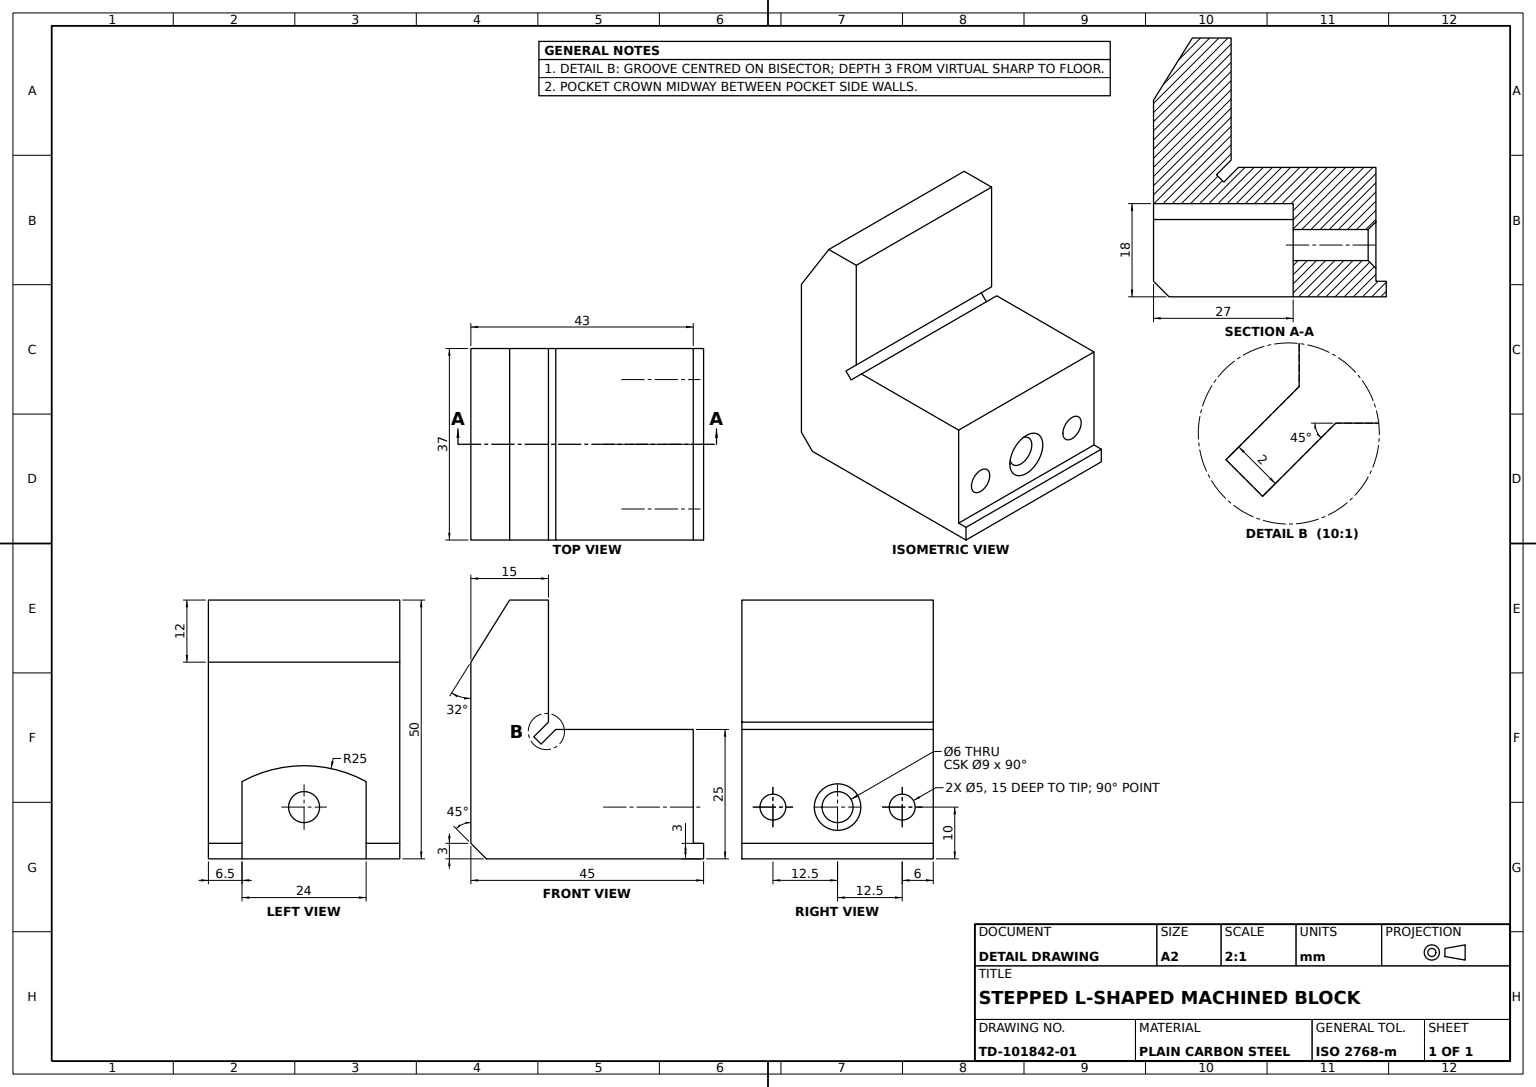
SolidWorks part; units mm, degrees
material "Plain Carbon Steel"
ref_plane "Front Plane" through (0, 0, 0) normal (0, 0, 1) x (1, 0, 0)
ref_plane "Top Plane" through (0, 0, 0) normal (0, 1, 0) x (1, 0, 0)
ref_plane "Right Plane" through (0, 0, 0) normal (1, 0, 0) x (0, 0, -1)
sketch "Block Profile Sketch" plane through (0, 0, 0) normal (0, 0, 1) x (1, 0, 0)
  line L0 (0, 0) -> (0, 13)
  line L1 (0, 13) -> (7.4984, 25)
  line L2 (7.4984, 25) -> (15, 25)
  line L3 (15, 25) -> (15, 0)
  line L4 (15, 0) -> (43, 0)
  line L5 (43, 0) -> (43, -22)
  line L6 (43, -22) -> (45, -22)
  line L7 (45, -22) -> (45, -25)
  line L8 (45, -25) -> (0, -25)
  line L9 (0, -25) -> (0, 0)
  dimension "D1" = 50
  dimension "D2" = 25
  dimension "D3" = 45
  dimension "D4" = 2
  dimension "D5" = 15
  dimension "D6" = 32
  dimension "D7" = 12
  dimension "D8" = 3
extrude "Anchor Block Body" add sketch "Block Profile Sketch" along normal mid plane 37
chamfer "Top Edge Chamfer 3x45" distance 3 angle 45 1 edges at (0, -25, 0)
sketch "Step Groove Sketch" plane through (0, 0, 18.5) normal (0, 0, 1) x (1, 0, 0)
  line L0 (15, 0) -> (12.8787, -2.1213) construction
  line L1 (15, 0) -> (17.4007, 2.4007) construction
  line L2 (15, 0) -> (15, 25) construction
  line L3 (12.8787, -2.1213) -> (12.1716, -1.4142)
  line L4 (12.1716, -1.4142) -> (15, 1.4142)
  line L5 (15, 1.4142) -> (16.4142, 0)
  line L6 (16.4142, 0) -> (13.5858, -2.8284)
  line L7 (13.5858, -2.8284) -> (12.8787, -2.1213)
  dimension "D1" = 45
  dimension "D2" = 3
  dimension "D3" = 2
extrude "Step Groove" cut sketch "Step Groove Sketch" against normal through all
sketch "Step Cut Sketch" plane through (0, 0, 0) normal (-1, 0, 0) x (0, 0, 1)
  line L0 (-12, -25) -> (-12, -10.0683)
  line L1 (18.5, -25) -> (-18.5, -25) construction
  line L2 (-12, -10.0683) -> (12, -10.0683) construction
  line L3 (12, -10.0683) -> (12, -25)
  line L4 (-12, -25) -> (12, -25)
  arc A0 (-12, -10.0683) -> (12, -10.0683) centre (0, -32) cw
  point P4 (0, -10.0683)
  point P9 (0, -7)
  dimension "D1" = 25
  dimension "D2" = 18
  dimension "D3" = 24
extrude "Step Cut 18 Deep" cut sketch "Step Cut Sketch" against normal offset from surface (27 mm away) 18 up to face at (45, -23.5, 0)
hole_wizard "Countersunk Thru Hole Ø6" positions "Sketch5" profile "Sketch6" hole size "Ø6.0" standard "DIN" end condition through all
sketch "Sketch5" plane through (43, 0, 0) normal (1, 0, 0) x (0, 0, -1)
  line L0 (-18.5, -25) -> (18.5, -25) construction
  point P0 (0, -15)
  dimension "D1" = 10
sketch "Sketch6" plane through (43, -15, 0) normal (0, 1, 0) x (0, 0, -1)
  line L0 (0, 0) -> (0, 43)
  line L1 (0, 43) -> (3, 43)
  line L2 (3, 43) -> (3, 1.5)
  line L3 (3, 1.5) -> (4.5, 0)
  line L5 (4.5, 0) -> (0, 0)
  line L6 (-3, 1.5) -> (-4.5, 0) construction
  line L11 (0, -6.35) -> (0, 107.95) construction
  dimension "Thru Hole Dia." = 6
  dimension "Thru Hole Depth" = 43
  dimension "Near C'Sink Dia." = 9
  dimension "Near C'Sink Angle" = 90
hole_wizard "Drilled Holes Ø5x15" positions "Sketch7" profile "Sketch8" hole size "Ø5.0" standard "DIN"
sketch "Sketch7" plane through (43, 0, 0) normal (1, 0, 0) x (0, 0, -1)
  line L0 (-18.5, -25) -> (18.5, -25) construction
  line L2 (0, 0) -> (0, -5.9875) construction
  point P0 (12.5, -15)
  point P2 (-12.5, -15)
  dimension "D1" = 10
  dimension "D2" = 25
sketch "Sketch8" plane through (43, -15, -12.5) normal (0, 1, 0) x (0, 0, -1)
  line L0 (0, 0) -> (0, 15)
  line L1 (0, 15) -> (2.5, 12.5)
  line L2 (2.5, 12.5) -> (2.5, 0)
  line L5 (2.5, 0) -> (0, 0)
  line L10 (0, 15) -> (-2.5, 12.5) construction
  line L11 (0, -6.35) -> (0, 107.95) construction
  dimension "Hole Dia." = 5
  dimension "Hole Depth" = 15
  dimension "Drill Angle" = 90
